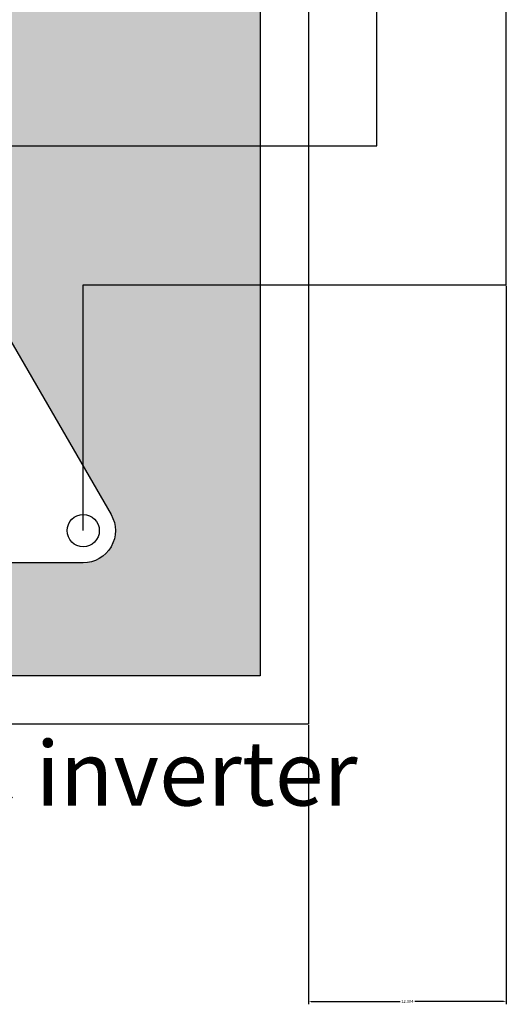
# Model space of a CAD drawing. Units: millimetres. Extents: x -8 to 285, y 5 to 221.
# Tile 18 of 30: x 241 to 271, y 5 to 66. Entities that reach past the tile are written whole.
import ezdxf

# ---------------------------------------------------------------- set-up
doc = ezdxf.new("R2010")
doc.units = ezdxf.units.MM
for name, color, linetype, lineweight in [('A-ANNO-DIMS', 2, 'Continuous', 18), ('E-ANNO-TEXT', 7, 'Continuous', 18), ('E-EQPM-PATT', 252, 'Continuous', 13), ('E-POWR-AC-NEUT', 3, 'Continuous', 25), ('E-POWR-INVR', 7, 'Continuous', 30)]:
    doc.layers.add(name, color=color, linetype=linetype, lineweight=lineweight)
doc.layers.add('E-POWR-AC-LINE', color=30, linetype='Continuous', lineweight=25, true_color=0xf26722)
doc.styles.get("Standard").update_dxf_attribs({"font": 'arial.ttf'})
doc.dimstyles.get("Standard").update_dxf_attribs({"dimtxt": 0.18, "dimasz": 0.18, "dimexe": 0.18, "dimexo": 0.0625, "dimgap": 0.09, "dimtad": 0, "dimtih": 1, "dimtoh": 1, "dimdec": 4, "dimzin": 0, "dimdsep": 46, "dimtxsty": 'Standard', "dimcen": 0.09, "dimadec": 0, "dimazin": 0, "dimtfac": 1, "dimtdec": 4, "dimtofl": 0, "dimtmove": 0, "dimatfit": 3, "dimfxl": 1, "dimtolj": 1, "dimtzin": 0, "dimarcsym": 0})

# ---------------------------------------------------------------- blocks, each defined once
blk = doc.blocks.new('*D27')
at = {"layer": 'A-ANNO-DIMS', "color": 0, "lineweight": -2, "transparency": 16777216}
for p, q in [((270.919, 49.862), (270.919, 5.222)), ((258.615, 22.567), (258.615, 5.222)), ((258.795, 5.402), (264.312, 5.402)), ((270.739, 5.402), (265.222, 5.402))]:
    blk.add_line(p, q, dxfattribs=at)
at = {"layer": 'A-ANNO-DIMS', "color": 0, "transparency": 16777216}
for points in [[(258.795, 5.432), (258.795, 5.372), (258.615, 5.402)], [(270.739, 5.432), (270.739, 5.372), (270.919, 5.402)]]:
    blk.add_solid(points, dxfattribs=at)
at = {"layer": 'Defpoints', "color": 0, "transparency": 16777216}
for p in [(270.919, 49.925), (258.615, 22.63), (270.919, 5.402)]:
    blk.add_point(p, dxfattribs=at)
at = {"layer": 'A-ANNO-DIMS', "color": 0, "transparency": 16777216, "insert": (264.767, 5.402), "char_height": 0.18, "attachment_point": 5}
blk.add_mtext('\\A1;12.304', dxfattribs=at)

msp = doc.modelspace()

# ---------------------------------------------------------------- hatches: boundary and pattern name
at = {"layer": 'E-EQPM-PATT'}
h = msp.add_hatch(color=256, dxfattribs=at)
h.set_gradient(color1=(175, 217, 170), color2=(175, 217, 170), tint=1)
h.paths.add_polyline_path([(255.6152, 99.7021), (190.9955, 99.7021), (190.9955, 53.4644), (215.8749, 53.4644), (215.8749, 47.6512), (217.2608, 47.6512), (219.2608, 45.6512), (219.2608, 32.6512), (199.2608, 32.6512), (199.2608, 44.4759), (190.9955, 44.4759), (190.9955, 28.2311), (237.8513, 28.2311), (237.8513, 32.6512), (231.5468, 32.6512, -0.5773503), (229.8147, 35.6512), (231.5468, 38.6512), (231.5468, 58.5666), (255.6152, 58.5666)])
h.paths.add_polyline_path([(208.2775, 92.6953), (238.0827, 92.6953), (238.0827, 67.6708), (208.2775, 67.6708)], flags=16)
h.paths.add_polyline_path([(213.1801, 80.183, -1), (233.1801, 80.183, -1)], flags=0)
h.paths.add_polyline_path([(215.1801, 80.183, -1), (231.1801, 80.183, -1)], flags=0)
h.paths.add_polyline_path([(217.1801, 80.183, -1), (229.1801, 80.183, -1)], flags=0)
h.paths.add_polyline_path([(219.1801, 80.183, -1), (227.1801, 80.183, -1)], flags=0)
h.paths.add_polyline_path([(255.6152, 58.5666), (231.5468, 58.5666), (231.5468, 38.6512), (236.3506, 46.9717, -0.5773503), (239.8147, 46.9717), (244.6186, 38.6512), (244.6186, 49.925), (255.6152, 49.925)], flags=17)
h.paths.add_polyline_path([(215.8749, 53.4644), (190.9955, 53.4644), (190.9955, 48.962), (202.4345, 48.962), (202.4345, 47.6512), (215.8749, 47.6512)], flags=17)
h.paths.add_polyline_path([(255.6152, 49.925), (244.6186, 49.925), (244.6186, 38.6512), (246.3506, 35.6512, -0.5773503), (244.6186, 32.6512), (237.8513, 32.6512), (237.8513, 28.2311), (190.9955, 28.2311), (190.9955, 25.6297), (255.6152, 25.6297)])
h.paths.add_polyline_path([(199.2608, 45.6512), (201.2608, 47.6512), (202.4345, 47.6512), (202.4345, 48.962), (190.9955, 48.962), (190.9955, 44.4759), (199.2608, 44.4759)], flags=17)

# ---------------------------------------------------------------- linework, layer by layer
at = {"layer": 'E-POWR-AC-LINE'}
msp.add_lwpolyline([(244.6186, 34.6512), (244.6186, 49.925), (270.9192, 49.925), (270.9192, 206.4568), (145.1651, 206.4568), (145.1651, 201.7939)], dxfattribs=at)
at = {"layer": 'E-POWR-AC-NEUT'}
msp.add_lwpolyline([(231.5468, 34.6512), (231.5468, 58.5666), (262.873, 58.5666), (262.873, 115.1427), (144.6762, 115.1427), (144.6762, 130.9614)], dxfattribs=at)
at = {"layer": 'E-POWR-INVR'}
for points in [[(187.9955, 102.7021), (258.6152, 102.7021), (258.6152, 22.6297), (187.9955, 22.6297)], [(190.9955, 99.7021), (255.6152, 99.7021), (255.6152, 25.6297), (190.9955, 25.6297)]]:
    msp.add_lwpolyline(points, close=True, dxfattribs=at)
msp.add_lwpolyline([(239.8147, 46.9717), (246.3506, 35.6512, -0.5773503), (244.6186, 32.6512), (231.5468, 32.6512, -0.5773503), (229.8147, 35.6512), (236.3506, 46.9717)], format="xyb", dxfattribs=at)
msp.add_circle((244.6186, 34.6512), 1, dxfattribs=at)

# ---------------------------------------------------------------- texts
at = {"layer": 'E-ANNO-TEXT', "insert": (194.1702, 21.5692), "char_height": 4, "attachment_point": 1}
msp.add_mtext_dynamic_manual_height_columns('120-230V DC to AC inverter', width=74.08228, gutter_width=12.5, heights=[0], dxfattribs=at)

# ---------------------------------------------------------------- dimensions: what is measured, and where the dimension line sits
at = {"layer": 'A-ANNO-DIMS'}
dim = msp.add_linear_dim(base=(270.9192, 5.402), p1=(258.6152, 22.6297), p2=(270.9192, 49.925), dimstyle='Standard', override={"dimdec": 3, "dimlfac": 1, "dimrnd": 0, "dimzin": 0, "dimdsep": 46, "dimlunit": 2}, dxfattribs=at)
dim.commit()
dim.dimension.update_dxf_attribs({"geometry": '*D27', "text_midpoint": (264.7672, 5.402)})

doc.saveas('drawing.dxf')
